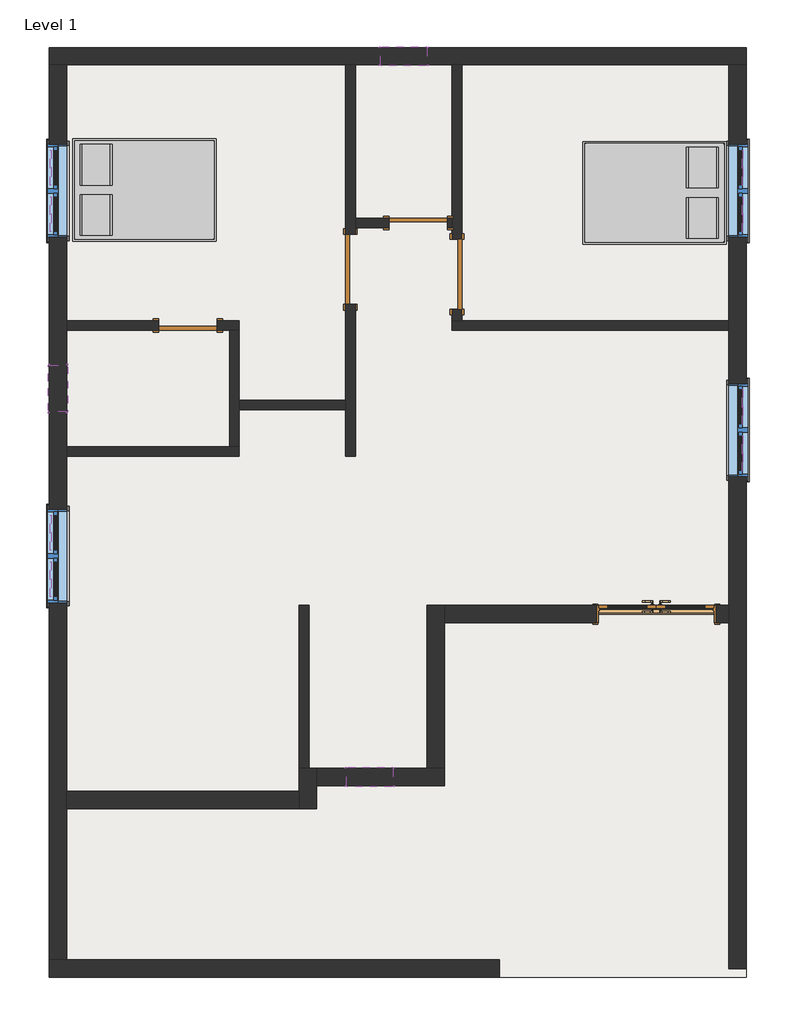
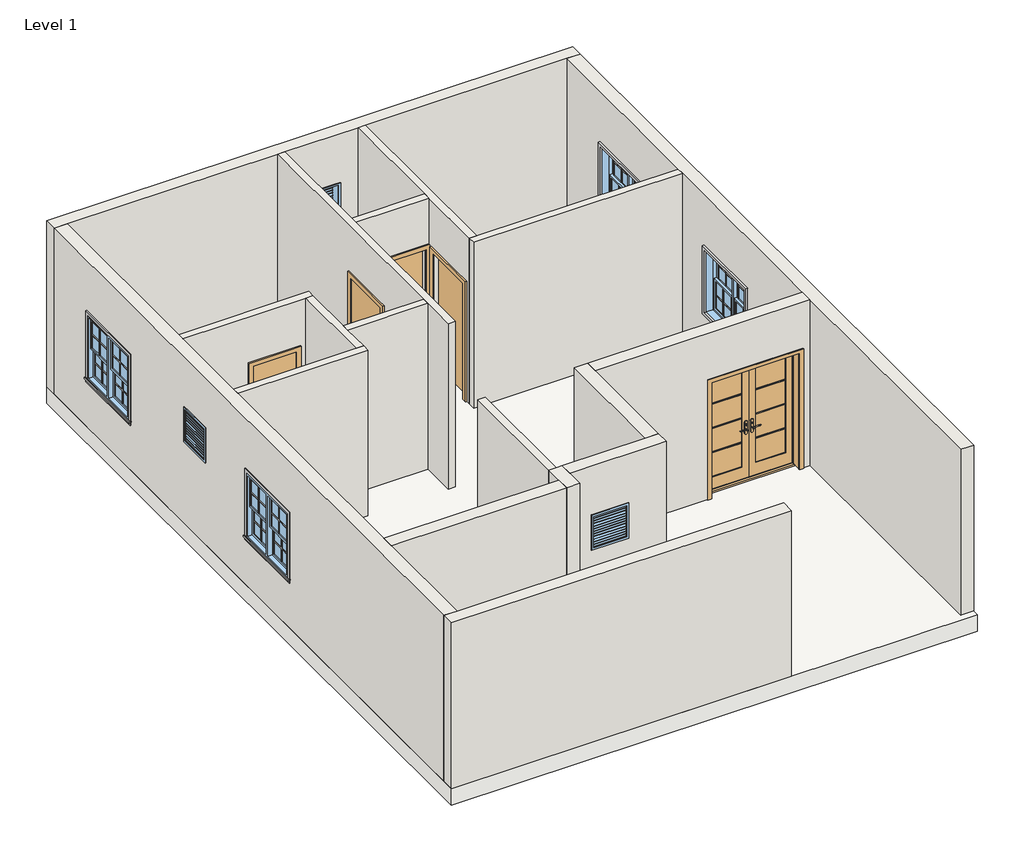
# One storey: 24 proxies, 18 walls, 7 windows, 5 doors, 2 furniture elements, 1 slab.
"""IFC4 building model written with IfcOpenShell, lengths in millimetres."""

from ifc_helpers import new_model, si_unit, frame, origin, origin_with_axes, place, context, project, spatial, polyline, outline, extrude, faceted_brep, transform, mapped, element, save
from components import muntin_pattern_2x2_muntin_pattern_2x2_3e1923be, muntin_pattern_2x2_muntin_pattern_2x2_6213a163, trim_window_exterior_flat_with_sill_91d32942, trim_window_exterior_flat_with_sill_c7d07f6c, trim_window_interior_flat_picture_frame_37b958cc, trim_window_interior_flat_picture_frame_8d0988b3, door_7ffae4ec, door_5304b0a0, door_0715e8d2, door_e36758a9, door_4d6c7550, bed_1_1346_x_1880mm_double_99e58f25, window_e23adcbe, window_25281ba2, window_f2d8fef0, window_407d3824

model = new_model("IFC4")

# Units and contexts
model_context = context("Model", 3, world=origin())
ifc_project = project(units=[si_unit("LENGTHUNIT", "METRE", prefix="MILLI")], contexts=[model_context])

# Site, building, storey
site = spatial("IfcSite", under=ifc_project)
building = spatial("IfcBuilding", under=site)
storey = spatial("IfcBuildingStorey", under=building, Name="Level 1", Elevation=0.0)

# Proxies
placement = place(None, origin())
muntin_pattern_2x2_muntin_pattern_2x2_shape = muntin_pattern_2x2_muntin_pattern_2x2_3e1923be(model_context)
element("IfcBuildingElementProxy", 1, Name="Muntin Pattern_2x2 : Muntin Pattern_2x2", ObjectType="Muntin Pattern_2x2 : Muntin Pattern_2x2", at=placement, inside=storey, context=model_context, shape_type="MappedRepresentation", body=[
    mapped(muntin_pattern_2x2_muntin_pattern_2x2_shape, transform((-10657.2556914, 7698.8778437, 1520.825), x_axis=(0.0, 1.0, 0.0), y_axis=(-1.0, 0.0, 0.0), z_axis=(0.0, 0.0, 1.0))),
])
element("IfcBuildingElementProxy", 2, Name="Muntin Pattern_2x2 : Muntin Pattern_2x2", ObjectType="Muntin Pattern_2x2 : Muntin Pattern_2x2", at=placement, inside=storey, context=model_context, shape_type="MappedRepresentation", body=[
    mapped(muntin_pattern_2x2_muntin_pattern_2x2_shape, transform((-10612.8056914, 7698.8778437, 990.6), x_axis=(0.0, 1.0, 0.0), y_axis=(-1.0, 0.0, 0.0), z_axis=(0.0, 0.0, 1.0))),
])
element("IfcBuildingElementProxy", 3, Name="Muntin Pattern_2x2 : Muntin Pattern_2x2", ObjectType="Muntin Pattern_2x2 : Muntin Pattern_2x2", at=placement, inside=storey, context=model_context, shape_type="MappedRepresentation", body=[
    mapped(muntin_pattern_2x2_muntin_pattern_2x2_shape, transform((-10657.2556914, 2910.9778437, 1520.825), x_axis=(0.0, 1.0, 0.0), y_axis=(-1.0, 0.0, 0.0), z_axis=(0.0, 0.0, 1.0))),
])
element("IfcBuildingElementProxy", 4, Name="Muntin Pattern_2x2 : Muntin Pattern_2x2", ObjectType="Muntin Pattern_2x2 : Muntin Pattern_2x2", at=placement, inside=storey, context=model_context, shape_type="MappedRepresentation", body=[
    mapped(muntin_pattern_2x2_muntin_pattern_2x2_shape, transform((-10612.8056914, 2910.9778437, 990.6), x_axis=(0.0, 1.0, 0.0), y_axis=(-1.0, 0.0, 0.0), z_axis=(0.0, 0.0, 1.0))),
])
element("IfcBuildingElementProxy", 5, Name="Muntin Pattern_2x2 : Muntin Pattern_2x2", ObjectType="Muntin Pattern_2x2 : Muntin Pattern_2x2", at=placement, inside=storey, context=model_context, shape_type="MappedRepresentation", body=[
    mapped(muntin_pattern_2x2_muntin_pattern_2x2_shape, transform((-1583.1056914, 3953.9653437, 1520.825), x_axis=(0.0, -1.0, 0.0), y_axis=(1.0, 0.0, 0.0), z_axis=(0.0, 0.0, 1.0))),
])
element("IfcBuildingElementProxy", 6, Name="Muntin Pattern_2x2 : Muntin Pattern_2x2", ObjectType="Muntin Pattern_2x2 : Muntin Pattern_2x2", at=placement, inside=storey, context=model_context, shape_type="MappedRepresentation", body=[
    mapped(muntin_pattern_2x2_muntin_pattern_2x2_shape, transform((-1627.5556914, 3953.9653437, 990.6), x_axis=(0.0, -1.0, 0.0), y_axis=(1.0, 0.0, 0.0), z_axis=(0.0, 0.0, 1.0))),
])
element("IfcBuildingElementProxy", 7, Name="Muntin Pattern_2x2 : Muntin Pattern_2x2", ObjectType="Muntin Pattern_2x2 : Muntin Pattern_2x2", at=placement, inside=storey, context=model_context, shape_type="MappedRepresentation", body=[
    mapped(muntin_pattern_2x2_muntin_pattern_2x2_shape, transform((-1583.1056914, 7090.8653437, 1520.825), x_axis=(0.0, -1.0, 0.0), y_axis=(1.0, 0.0, 0.0), z_axis=(0.0, 0.0, 1.0))),
])
element("IfcBuildingElementProxy", 8, Name="Muntin Pattern_2x2 : Muntin Pattern_2x2", ObjectType="Muntin Pattern_2x2 : Muntin Pattern_2x2", at=placement, inside=storey, context=model_context, shape_type="MappedRepresentation", body=[
    mapped(muntin_pattern_2x2_muntin_pattern_2x2_shape, transform((-1627.5556914, 7090.8653437, 990.6), x_axis=(0.0, -1.0, 0.0), y_axis=(1.0, 0.0, 0.0), z_axis=(0.0, 0.0, 1.0))),
])
muntin_pattern_2x2_muntin_pattern_2x2_2_shape = muntin_pattern_2x2_muntin_pattern_2x2_6213a163(model_context)
element("IfcBuildingElementProxy", 9, Name="Muntin Pattern_2x2 : Muntin Pattern_2x2", ObjectType="Muntin Pattern_2x2 : Muntin Pattern_2x2", at=placement, inside=storey, context=model_context, shape_type="MappedRepresentation", body=[
    mapped(muntin_pattern_2x2_muntin_pattern_2x2_2_shape, transform((-10657.2556914, 7090.8653437, 1520.825), x_axis=(0.0, -1.0, 0.0), y_axis=(1.0, 0.0, 0.0), z_axis=(0.0, 0.0, 1.0))),
])
element("IfcBuildingElementProxy", 10, Name="Muntin Pattern_2x2 : Muntin Pattern_2x2", ObjectType="Muntin Pattern_2x2 : Muntin Pattern_2x2", at=placement, inside=storey, context=model_context, shape_type="MappedRepresentation", body=[
    mapped(muntin_pattern_2x2_muntin_pattern_2x2_2_shape, transform((-10612.8056914, 7090.8653437, 990.6), x_axis=(0.0, -1.0, 0.0), y_axis=(1.0, 0.0, 0.0), z_axis=(0.0, 0.0, 1.0))),
])
element("IfcBuildingElementProxy", 11, Name="Muntin Pattern_2x2 : Muntin Pattern_2x2", ObjectType="Muntin Pattern_2x2 : Muntin Pattern_2x2", at=placement, inside=storey, context=model_context, shape_type="MappedRepresentation", body=[
    mapped(muntin_pattern_2x2_muntin_pattern_2x2_2_shape, transform((-10657.2556914, 2302.9653437, 1520.825), x_axis=(0.0, -1.0, 0.0), y_axis=(1.0, 0.0, 0.0), z_axis=(0.0, 0.0, 1.0))),
])
element("IfcBuildingElementProxy", 12, Name="Muntin Pattern_2x2 : Muntin Pattern_2x2", ObjectType="Muntin Pattern_2x2 : Muntin Pattern_2x2", at=placement, inside=storey, context=model_context, shape_type="MappedRepresentation", body=[
    mapped(muntin_pattern_2x2_muntin_pattern_2x2_2_shape, transform((-10612.8056914, 2302.9653437, 990.6), x_axis=(0.0, -1.0, 0.0), y_axis=(1.0, 0.0, 0.0), z_axis=(0.0, 0.0, 1.0))),
])
element("IfcBuildingElementProxy", 13, Name="Muntin Pattern_2x2 : Muntin Pattern_2x2", ObjectType="Muntin Pattern_2x2 : Muntin Pattern_2x2", at=placement, inside=storey, context=model_context, shape_type="MappedRepresentation", body=[
    mapped(muntin_pattern_2x2_muntin_pattern_2x2_2_shape, transform((-1583.1056914, 4561.9778437, 1520.825), x_axis=(0.0, 1.0, 0.0), y_axis=(-1.0, 0.0, 0.0), z_axis=(0.0, 0.0, 1.0))),
])
element("IfcBuildingElementProxy", 14, Name="Muntin Pattern_2x2 : Muntin Pattern_2x2", ObjectType="Muntin Pattern_2x2 : Muntin Pattern_2x2", at=placement, inside=storey, context=model_context, shape_type="MappedRepresentation", body=[
    mapped(muntin_pattern_2x2_muntin_pattern_2x2_2_shape, transform((-1627.5556914, 4561.9778437, 990.6), x_axis=(0.0, 1.0, 0.0), y_axis=(-1.0, 0.0, 0.0), z_axis=(0.0, 0.0, 1.0))),
])
element("IfcBuildingElementProxy", 15, Name="Muntin Pattern_2x2 : Muntin Pattern_2x2", ObjectType="Muntin Pattern_2x2 : Muntin Pattern_2x2", at=placement, inside=storey, context=model_context, shape_type="MappedRepresentation", body=[
    mapped(muntin_pattern_2x2_muntin_pattern_2x2_2_shape, transform((-1583.1056914, 7698.8778437, 1520.825), x_axis=(0.0, 1.0, 0.0), y_axis=(-1.0, 0.0, 0.0), z_axis=(0.0, 0.0, 1.0))),
])
element("IfcBuildingElementProxy", 16, Name="Muntin Pattern_2x2 : Muntin Pattern_2x2", ObjectType="Muntin Pattern_2x2 : Muntin Pattern_2x2", at=placement, inside=storey, context=model_context, shape_type="MappedRepresentation", body=[
    mapped(muntin_pattern_2x2_muntin_pattern_2x2_2_shape, transform((-1627.5556914, 7698.8778437, 990.6), x_axis=(0.0, 1.0, 0.0), y_axis=(-1.0, 0.0, 0.0), z_axis=(0.0, 0.0, 1.0))),
])
trim_window_exterior_flat_with_sill_shape = trim_window_exterior_flat_with_sill_91d32942(model_context)
element("IfcBuildingElementProxy", 17, Name="Trim-Window-Exterior-Flat : with Sill", ObjectType="Trim-Window-Exterior-Flat : with Sill", at=placement, inside=storey, context=model_context, shape_type="MappedRepresentation", body=[
    mapped(trim_window_exterior_flat_with_sill_shape, transform((-1548.1806914, 7394.8715937, 2082.8), x_axis=(0.0, 1.0, 0.0), y_axis=(0.0, 0.0, 1.0), z_axis=(1.0, 0.0, 0.0))),
])
trim_window_exterior_flat_with_sill_2_shape = trim_window_exterior_flat_with_sill_c7d07f6c(model_context)
element("IfcBuildingElementProxy", 18, Name="Trim-Window-Exterior-Flat : with Sill", ObjectType="Trim-Window-Exterior-Flat : with Sill", at=placement, inside=storey, context=model_context, shape_type="MappedRepresentation", body=[
    mapped(trim_window_exterior_flat_with_sill_2_shape, transform((-10692.1806914, 7394.8715937, 2082.8), x_axis=(0.0, 1.0, 0.0), y_axis=(0.0, 0.0, -1.0), z_axis=(-1.0, 0.0, 0.0))),
])
element("IfcBuildingElementProxy", 19, Name="Trim-Window-Exterior-Flat : with Sill", ObjectType="Trim-Window-Exterior-Flat : with Sill", at=placement, inside=storey, context=model_context, shape_type="MappedRepresentation", body=[
    mapped(trim_window_exterior_flat_with_sill_2_shape, transform((-10692.1806914, 2606.9715937, 2082.8), x_axis=(0.0, 1.0, 0.0), y_axis=(0.0, 0.0, -1.0), z_axis=(-1.0, 0.0, 0.0))),
])
element("IfcBuildingElementProxy", 20, Name="Trim-Window-Exterior-Flat : with Sill", ObjectType="Trim-Window-Exterior-Flat : with Sill", at=placement, inside=storey, context=model_context, shape_type="MappedRepresentation", body=[
    mapped(trim_window_exterior_flat_with_sill_2_shape, transform((-1548.1806914, 4257.9715937, 2082.8), x_axis=(0.0, -1.0, 0.0), y_axis=(0.0, 0.0, -1.0), z_axis=(1.0, 0.0, 0.0))),
])
trim_window_interior_flat_picture_frame_shape = trim_window_interior_flat_picture_frame_37b958cc(model_context)
element("IfcBuildingElementProxy", 21, Name="Trim-Window-Interior-Flat : Picture Frame", ObjectType="Trim-Window-Interior-Flat : Picture Frame", at=placement, inside=storey, context=model_context, shape_type="MappedRepresentation", body=[
    mapped(trim_window_interior_flat_picture_frame_shape, transform((-1776.7806914, 7394.8715937, 2082.8), x_axis=(0.0, -1.0, 0.0), y_axis=(0.0, 0.0, 1.0), z_axis=(-1.0, 0.0, 0.0))),
])
trim_window_interior_flat_picture_frame_2_shape = trim_window_interior_flat_picture_frame_8d0988b3(model_context)
element("IfcBuildingElementProxy", 22, Name="Trim-Window-Interior-Flat : Picture Frame", ObjectType="Trim-Window-Interior-Flat : Picture Frame", at=placement, inside=storey, context=model_context, shape_type="MappedRepresentation", body=[
    mapped(trim_window_interior_flat_picture_frame_2_shape, transform((-10463.5806914, 7394.8715937, 2082.8), x_axis=(0.0, -1.0, 0.0), y_axis=(0.0, 0.0, -1.0), z_axis=(1.0, 0.0, 0.0))),
])
element("IfcBuildingElementProxy", 23, Name="Trim-Window-Interior-Flat : Picture Frame", ObjectType="Trim-Window-Interior-Flat : Picture Frame", at=placement, inside=storey, context=model_context, shape_type="MappedRepresentation", body=[
    mapped(trim_window_interior_flat_picture_frame_2_shape, transform((-10463.5806914, 2606.9715937, 2082.8), x_axis=(0.0, -1.0, 0.0), y_axis=(0.0, 0.0, -1.0), z_axis=(1.0, 0.0, 0.0))),
])
element("IfcBuildingElementProxy", 24, Name="Trim-Window-Interior-Flat : Picture Frame", ObjectType="Trim-Window-Interior-Flat : Picture Frame", at=placement, inside=storey, context=model_context, shape_type="MappedRepresentation", body=[
    mapped(trim_window_interior_flat_picture_frame_2_shape, transform((-1776.7806914, 4257.9715937, 2082.8), x_axis=(0.0, 1.0, 0.0), y_axis=(0.0, 0.0, -1.0), z_axis=(-1.0, 0.0, 0.0))),
])

# Doors
door_shape = door_7ffae4ec(model_context)
element("IfcDoor", 25, ObjectType="Door-Exterior-Double-Full Glass-Wood_Clad : 60\" x 84\"", at=placement, inside=storey, context=model_context, shape_type="MappedRepresentation", body=[
    mapped(door_shape, transform((-2729.2806914, 1848.1465937, 0.0), x_axis=(1.0, 0.0, 0.0), y_axis=(0.0, 1.0, 0.0), z_axis=(0.0, 0.0, 1.0))),
])
door_2_shape = door_5304b0a0(model_context)
element("IfcDoor", 26, ObjectType="Door-Single-Panel : 36\" x 84\"", at=placement, inside=storey, context=model_context, shape_type="MappedRepresentation", body=[
    mapped(door_2_shape, transform((-6742.4806914, 6366.1715937, 0.0), x_axis=(0.0, -1.0, 0.0), y_axis=(1.0, 0.0, 0.0), z_axis=(0.0, 0.0, 1.0))),
])
door_3_shape = door_0715e8d2(model_context)
element("IfcDoor", 27, ObjectType="Door-Single-Panel : 36\" x 84\"", at=placement, inside=storey, context=model_context, shape_type="MappedRepresentation", body=[
    mapped(door_3_shape, transform((-5345.4806914, 6302.6715937, 0.0), x_axis=(0.0, -1.0, 0.0), y_axis=(1.0, 0.0, 0.0), z_axis=(0.0, 0.0, 1.0))),
])
door_4_shape = door_e36758a9(model_context)
element("IfcDoor", 28, ObjectType="Single-Flush : 30\" x 84\"", at=placement, inside=storey, context=model_context, shape_type="MappedRepresentation", body=[
    mapped(door_4_shape, transform((-8876.0806914, 5629.5715937, 0.0), x_axis=(1.0, 0.0, 0.0), y_axis=(0.0, 1.0, 0.0), z_axis=(0.0, 0.0, 1.0))),
])
door_5_shape = door_4d6c7550(model_context)
element("IfcDoor", 29, ObjectType="Single-Flush : 30\" x 84\"", at=placement, inside=storey, context=model_context, shape_type="MappedRepresentation", body=[
    mapped(door_5_shape, transform((-5853.4806914, 6975.7715937, 0.0), x_axis=(1.0, 0.0, 0.0), y_axis=(0.0, 1.0, 0.0), z_axis=(0.0, 0.0, 1.0))),
])

# Furniture
bed_1_1346_x_1880mm_double_shape = bed_1_1346_x_1880mm_double_99e58f25(model_context)
element("IfcFurniture", 30, ObjectType="Bed (1) : 1346 x 1880mm - Double", at=placement, inside=storey, context=model_context, shape_type="MappedRepresentation", body=[
    mapped(bed_1_1346_x_1880mm_double_shape, transform((-2520.4511832, 7708.5240527, 0.0), x_axis=(0.0, -1.0, 0.0), y_axis=(1.0, 0.0, 0.0), z_axis=(0.0, 0.0, 1.0))),
])
element("IfcFurniture", 31, ObjectType="Bed (1) : 1346 x 1880mm - Double", at=placement, inside=storey, context=model_context, shape_type="MappedRepresentation", body=[
    mapped(bed_1_1346_x_1880mm_double_shape, transform((-9681.8101996, 7068.5191346, 0.0), x_axis=(0.0, 1.0, 0.0), y_axis=(-1.0, 0.0, 0.0), z_axis=(0.0, 0.0, 1.0))),
])

# Slab
element("IfcSlab", 32, ObjectType="Generic - 12\"", at=placement, inside=storey, context=model_context, shape_type="SweptSolid", body=[
    extrude(outline(polyline([(-10692.1806914, 9274.4715937), (-1548.1806914, 9274.4715937), (-1548.1806914, -2917.5284063), (-10692.1806914, -2917.5284063), (-10692.1806914, 9274.4715937)])), frame((0.0, 0.0, -304.8), z_axis=(0.0, 0.0, 1.0), x_axis=(1.0, 0.0, 0.0)), (0.0, 0.0, 1.0), 304.8),
])

# Walls
element("IfcWall", 33, ObjectType="Generic - 5\"", at=placement, inside=storey, context=model_context, shape_type="Brep", body=[
    faceted_brep([(-8495.0806914, 5566.0715937, 2133.6), (-8495.0806914, 5566.0715937, 0.0), (-8329.9806914, 5566.0715937, 0.0), (-8202.9806914, 5566.0715937, 0.0), (-8202.9806914, 5566.0715937, 3048.0), (-8329.9806914, 5566.0715937, 3048.0), (-10463.5806914, 5566.0715937, 3048.0), (-10463.5806914, 5566.0715937, 0.0), (-9257.0806914, 5566.0715937, 0.0), (-9257.0806914, 5566.0715937, 2133.6), (-8202.9806914, 5693.0715937, 0.0), (-8495.0806914, 5693.0715937, 0.0), (-8495.0806914, 5693.0715937, 2133.6), (-9257.0806914, 5693.0715937, 2133.6), (-9257.0806914, 5693.0715937, 0.0), (-10463.5806914, 5693.0715937, 0.0), (-10463.5806914, 5693.0715937, 3048.0), (-8202.9806914, 5693.0715937, 3048.0)], [[[0, 1, 2, 3, 4, 5, 6, 7, 8, 9]], [[10, 11, 12, 13, 14, 15, 16, 17]], [[8, 7, 15, 14]], [[3, 2, 1, 11, 10]], [[6, 5, 4, 17, 16]], [[7, 6, 16, 15]], [[4, 3, 10, 17]], [[12, 11, 1, 0]], [[13, 12, 0, 9]], [[14, 13, 9, 8]]]),
])
element("IfcWall", 34, ObjectType="Generic - 5\"", at=placement, inside=storey, context=model_context, shape_type="Brep", body=[
    faceted_brep([(-6805.9806914, 5908.9715937, 2133.6), (-6805.9806914, 5908.9715937, 0.0), (-6805.9806914, 4651.6715937, 0.0), (-6805.9806914, 4524.6715937, 0.0), (-6805.9806914, 3915.0715937, 0.0), (-6805.9806914, 3915.0715937, 3048.0), (-6805.9806914, 4524.6715937, 3048.0), (-6805.9806914, 4651.6715937, 3048.0), (-6805.9806914, 9045.8715937, 3048.0), (-6805.9806914, 9045.8715937, 0.0), (-6805.9806914, 6823.3715937, 0.0), (-6805.9806914, 6823.3715937, 2133.6), (-6678.9806914, 3915.0715937, 0.0), (-6678.9806914, 5908.9715937, 0.0), (-6678.9806914, 5908.9715937, 2133.6), (-6678.9806914, 6823.3715937, 2133.6), (-6678.9806914, 6823.3715937, 0.0), (-6678.9806914, 6912.2715937, 0.0), (-6678.9806914, 7039.2715937, 0.0), (-6678.9806914, 9045.8715937, 0.0), (-6678.9806914, 9045.8715937, 3048.0), (-6678.9806914, 7039.2715937, 3048.0), (-6678.9806914, 6912.2715937, 3048.0), (-6678.9806914, 3915.0715937, 3048.0)], [[[0, 1, 2, 3, 4, 5, 6, 7, 8, 9, 10, 11]], [[12, 13, 14, 15, 16, 17, 18, 19, 20, 21, 22, 23]], [[10, 9, 19, 18, 17, 16]], [[4, 3, 2, 1, 13, 12]], [[5, 4, 12, 23]], [[8, 7, 6, 5, 23, 22, 21, 20]], [[9, 8, 20, 19]], [[14, 13, 1, 0]], [[15, 14, 0, 11]], [[16, 15, 11, 10]]]),
])
element("IfcWall", 35, ObjectType="Generic - 5\"", at=placement, inside=storey, context=model_context, shape_type="SweptSolid", body=[
    extrude(outline(polyline([(2133.6, -5472.4806914), (0.0, -5472.4806914), (0.0, -5408.9806914), (3048.0, -5408.9806914), (3048.0, -6678.9806914), (0.0, -6678.9806914), (0.0, -6234.4806914), (2133.6, -6234.4806914), (2133.6, -5472.4806914)])), frame((0.0, 6912.2715937, 0.0), z_axis=(0.0, 1.0, 0.0), x_axis=(0.0, 0.0, 1.0)), (0.0, 0.0, 1.0), 127.0),
])
element("IfcWall", 36, ObjectType="Generic - 5\"", at=placement, inside=storey, context=model_context, shape_type="Brep", body=[
    faceted_brep([(-5281.9806914, 5693.0715937, 0.0), (-5281.9806914, 5845.4715937, 0.0), (-5281.9806914, 5845.4715937, 2133.6), (-5281.9806914, 6759.8715937, 2133.6), (-5281.9806914, 6759.8715937, 0.0), (-5281.9806914, 9045.8715937, 0.0), (-5281.9806914, 9045.8715937, 3048.0), (-5281.9806914, 5693.0715937, 3048.0), (-5408.9806914, 5845.4715937, 2133.6), (-5408.9806914, 5845.4715937, 0.0), (-5408.9806914, 5693.0715937, 0.0), (-5408.9806914, 5693.0715937, 3048.0), (-5408.9806914, 6912.2715937, 3048.0), (-5408.9806914, 7039.2715937, 3048.0), (-5408.9806914, 9045.8715937, 3048.0), (-5408.9806914, 9045.8715937, 0.0), (-5408.9806914, 7039.2715937, 0.0), (-5408.9806914, 6912.2715937, 0.0), (-5408.9806914, 6759.8715937, 0.0), (-5408.9806914, 6759.8715937, 2133.6)], [[[0, 1, 2, 3, 4, 5, 6, 7]], [[8, 9, 10, 11, 12, 13, 14, 15, 16, 17, 18, 19]], [[10, 9, 1, 0]], [[18, 17, 16, 15, 5, 4]], [[7, 6, 14, 13, 12, 11]], [[6, 5, 15, 14]], [[0, 7, 11, 10]], [[2, 1, 9, 8]], [[3, 2, 8, 19]], [[4, 3, 19, 18]]]),
])
element("IfcWall", 37, ObjectType="Generic - 5\"", at=placement, inside=storey, context=model_context, shape_type="Brep", body=[
    faceted_brep([(-1776.7806914, 5693.0715937, 0.0), (-5281.9806914, 5693.0715937, 0.0), (-5408.9806914, 5693.0715937, 0.0), (-5408.9806914, 5693.0715937, 3048.0), (-5281.9806914, 5693.0715937, 3048.0), (-1776.7806914, 5693.0715937, 3048.0), (-1776.7806914, 5566.0715937, 0.0), (-1776.7806914, 5566.0715937, 3048.0), (-5408.9806914, 5566.0715937, 3048.0), (-5408.9806914, 5566.0715937, 0.0)], [[[0, 1, 2, 3, 4, 5]], [[6, 7, 8, 9]], [[2, 1, 0, 6, 9]], [[5, 4, 3, 8, 7]], [[0, 5, 7, 6]], [[3, 2, 9, 8]]]),
])
element("IfcWall", 38, ObjectType="Generic - 5\"", at=placement, inside=storey, context=model_context, shape_type="Brep", body=[
    faceted_brep([(-10463.5806914, 3915.0715937, 0.0), (-8202.9806914, 3915.0715937, 0.0), (-8202.9806914, 3915.0715937, 3048.0), (-10463.5806914, 3915.0715937, 3048.0), (-10463.5806914, 4042.0715937, 0.0), (-10463.5806914, 4042.0715937, 3048.0), (-8329.9806914, 4042.0715937, 3048.0), (-8202.9806914, 4042.0715937, 3048.0), (-8202.9806914, 4042.0715937, 0.0), (-8329.9806914, 4042.0715937, 0.0)], [[[0, 1, 2, 3]], [[4, 5, 6, 7, 8, 9]], [[1, 0, 4, 9, 8]], [[3, 2, 7, 6, 5]], [[0, 3, 5, 4]], [[2, 1, 8, 7]]]),
])
element("IfcWall", 39, ObjectType="Generic - 5\"", at=placement, inside=storey, context=model_context, shape_type="Brep", body=[
    faceted_brep([(-8329.9806914, 5566.0715937, 0.0), (-8329.9806914, 4042.0715937, 0.0), (-8329.9806914, 4042.0715937, 3048.0), (-8329.9806914, 5566.0715937, 3048.0), (-8202.9806914, 5566.0715937, 0.0), (-8202.9806914, 5566.0715937, 3048.0), (-8202.9806914, 4651.6715937, 3048.0), (-8202.9806914, 4524.6715937, 3048.0), (-8202.9806914, 4042.0715937, 3048.0), (-8202.9806914, 4042.0715937, 0.0), (-8202.9806914, 4524.6715937, 0.0), (-8202.9806914, 4651.6715937, 0.0)], [[[0, 1, 2, 3]], [[4, 5, 6, 7, 8, 9, 10, 11]], [[1, 0, 4, 11, 10, 9]], [[3, 2, 8, 7, 6, 5]], [[0, 3, 5, 4]], [[2, 1, 9, 8]]]),
])
element("IfcWall", 40, ObjectType="Generic - 5\"", at=placement, inside=storey, context=model_context, shape_type="SweptSolid", body=[
    extrude(outline(polyline([(-6805.9806914, 4524.6715937), (-8202.9806914, 4524.6715937), (-8202.9806914, 4651.6715937), (-6805.9806914, 4651.6715937), (-6805.9806914, 4524.6715937)])), origin_with_axes(), (0.0, 0.0, 1.0), 3048.0),
])
element("IfcWall", 41, ObjectType="Generic - 5\"", at=placement, inside=storey, context=model_context, shape_type="SweptSolid", body=[
    extrude(outline(polyline([(-7415.5806914, -174.3284063), (-7415.5806914, 1959.2715937), (-7288.5806914, 1959.2715937), (-7288.5806914, -174.3284063), (-7415.5806914, -174.3284063)])), origin_with_axes(), (0.0, 0.0, 1.0), 3048.0),
])
element("IfcWall", 42, ObjectType="Generic - 9\"", at=placement, inside=storey, context=model_context, shape_type="Brep", body=[
    faceted_brep([(-10692.1806914, 9045.8715937, 0.0), (-10463.5806914, 9045.8715937, 0.0), (-6805.9806914, 9045.8715937, 0.0), (-6678.9806914, 9045.8715937, 0.0), (-5408.9806914, 9045.8715937, 0.0), (-5281.9806914, 9045.8715937, 0.0), (-1776.7806914, 9045.8715937, 0.0), (-1548.1806914, 9045.8715937, 0.0), (-1548.1806914, 9045.8715937, 3048.0), (-1776.7806914, 9045.8715937, 3048.0), (-5281.9806914, 9045.8715937, 3048.0), (-5408.9806914, 9045.8715937, 3048.0), (-6678.9806914, 9045.8715937, 3048.0), (-6805.9806914, 9045.8715937, 3048.0), (-10463.5806914, 9045.8715937, 3048.0), (-10692.1806914, 9045.8715937, 3048.0), (-5739.1806914, 9045.8715937, 2133.6), (-5739.1806914, 9045.8715937, 1524.0), (-6348.7806914, 9045.8715937, 1524.0), (-6348.7806914, 9045.8715937, 2133.6), (-10692.1806914, 9274.4715937, 0.0), (-10692.1806914, 9274.4715937, 3048.0), (-1548.1806914, 9274.4715937, 3048.0), (-1548.1806914, 9274.4715937, 0.0), (-5739.1806914, 9274.4715937, 2133.6), (-6348.7806914, 9274.4715937, 2133.6), (-6348.7806914, 9274.4715937, 1524.0), (-5739.1806914, 9274.4715937, 1524.0)], [[[0, 1, 2, 3, 4, 5, 6, 7, 8, 9, 10, 11, 12, 13, 14, 15], [16, 17, 18, 19]], [[20, 21, 22, 23], [24, 25, 26, 27]], [[7, 6, 5, 4, 3, 2, 1, 0, 20, 23]], [[15, 14, 13, 12, 11, 10, 9, 8, 22, 21]], [[8, 7, 23, 22]], [[0, 15, 21, 20]], [[17, 16, 24, 27]], [[18, 17, 27, 26]], [[19, 18, 26, 25]], [[16, 19, 25, 24]]]),
])
element("IfcWall", 43, ObjectType="Generic - 9\"", at=placement, inside=storey, context=model_context, shape_type="Brep", body=[
    faceted_brep([(-1776.7806914, 9045.8715937, 0.0), (-1776.7806914, 5693.0715937, 0.0), (-1776.7806914, 5566.0715937, 0.0), (-1776.7806914, 1959.2715937, 0.0), (-1776.7806914, 1730.6715937, 0.0), (-1776.7806914, -2803.2284063, 0.0), (-1776.7806914, -2803.2284063, 3048.0), (-1776.7806914, 1730.6715937, 3048.0), (-1776.7806914, 1959.2715937, 3048.0), (-1776.7806914, 5566.0715937, 3048.0), (-1776.7806914, 5693.0715937, 3048.0), (-1776.7806914, 9045.8715937, 3048.0), (-1776.7806914, 3648.3715937, 2082.8), (-1776.7806914, 3648.3715937, 914.4), (-1776.7806914, 4867.5715937, 914.4), (-1776.7806914, 4867.5715937, 2082.8), (-1776.7806914, 8004.4715937, 2082.8), (-1776.7806914, 6785.2715937, 2082.8), (-1776.7806914, 6785.2715937, 914.4), (-1776.7806914, 8004.4715937, 914.4), (-1548.1806914, 9045.8715937, 0.0), (-1548.1806914, 9045.8715937, 3048.0), (-1548.1806914, -2803.2284063, 3048.0), (-1548.1806914, -2803.2284063, 0.0), (-1548.1806914, 3648.3715937, 2082.8), (-1548.1806914, 4867.5715937, 2082.8), (-1548.1806914, 4867.5715937, 914.4), (-1548.1806914, 3648.3715937, 914.4), (-1548.1806914, 8004.4715937, 2082.8), (-1548.1806914, 8004.4715937, 914.4), (-1548.1806914, 6785.2715937, 914.4), (-1548.1806914, 6785.2715937, 2082.8)], [[[0, 1, 2, 3, 4, 5, 6, 7, 8, 9, 10, 11], [12, 13, 14, 15], [16, 17, 18, 19]], [[20, 21, 22, 23], [24, 25, 26, 27], [28, 29, 30, 31]], [[5, 4, 3, 2, 1, 0, 20, 23]], [[6, 5, 23, 22]], [[11, 10, 9, 8, 7, 6, 22, 21]], [[0, 11, 21, 20]], [[13, 12, 24, 27]], [[14, 13, 27, 26]], [[15, 14, 26, 25]], [[12, 15, 25, 24]], [[29, 28, 16, 19]], [[30, 29, 19, 18]], [[31, 30, 18, 17]], [[28, 31, 17, 16]]]),
])
element("IfcWall", 44, ObjectType="Generic - 9\"", at=placement, inside=storey, context=model_context, shape_type="Brep", body=[
    faceted_brep([(-4786.6806914, -2688.9284063, 0.0), (-10463.5806914, -2688.9284063, 0.0), (-10692.1806914, -2688.9284063, 0.0), (-10692.1806914, -2688.9284063, 3048.0), (-10463.5806914, -2688.9284063, 3048.0), (-4786.6806914, -2688.9284063, 3048.0), (-4786.6806914, -2917.5284063, 0.0), (-4786.6806914, -2917.5284063, 3048.0), (-10692.1806914, -2917.5284063, 3048.0), (-10692.1806914, -2917.5284063, 0.0)], [[[0, 1, 2, 3, 4, 5]], [[6, 7, 8, 9]], [[2, 1, 0, 6, 9]], [[5, 4, 3, 8, 7]], [[0, 5, 7, 6]], [[3, 2, 9, 8]]]),
])
element("IfcWall", 45, ObjectType="Generic - 9\"", at=placement, inside=storey, context=model_context, shape_type="Brep", body=[
    faceted_brep([(-10463.5806914, -2688.9284063, 0.0), (-10463.5806914, -707.7284063, 0.0), (-10463.5806914, -479.1284063, 0.0), (-10463.5806914, 3915.0715937, 0.0), (-10463.5806914, 4042.0715937, 0.0), (-10463.5806914, 5566.0715937, 0.0), (-10463.5806914, 5693.0715937, 0.0), (-10463.5806914, 9045.8715937, 0.0), (-10463.5806914, 9045.8715937, 3048.0), (-10463.5806914, 5693.0715937, 3048.0), (-10463.5806914, 5566.0715937, 3048.0), (-10463.5806914, 4042.0715937, 3048.0), (-10463.5806914, 3915.0715937, 3048.0), (-10463.5806914, -479.1284063, 3048.0), (-10463.5806914, -707.7284063, 3048.0), (-10463.5806914, -2688.9284063, 3048.0), (-10463.5806914, 8004.4715937, 2082.8), (-10463.5806914, 8004.4715937, 914.4), (-10463.5806914, 6785.2715937, 914.4), (-10463.5806914, 6785.2715937, 2082.8), (-10463.5806914, 3216.5715937, 2082.8), (-10463.5806914, 3216.5715937, 914.4), (-10463.5806914, 1997.3715937, 914.4), (-10463.5806914, 1997.3715937, 2082.8), (-10463.5806914, 4499.2715937, 2133.6), (-10463.5806914, 5108.8715937, 2133.6), (-10463.5806914, 5108.8715937, 1524.0), (-10463.5806914, 4499.2715937, 1524.0), (-10692.1806914, -2688.9284063, 0.0), (-10692.1806914, -2688.9284063, 3048.0), (-10692.1806914, 9045.8715937, 3048.0), (-10692.1806914, 9045.8715937, 0.0), (-10692.1806914, 8004.4715937, 2082.8), (-10692.1806914, 6785.2715937, 2082.8), (-10692.1806914, 6785.2715937, 914.4), (-10692.1806914, 8004.4715937, 914.4), (-10692.1806914, 3216.5715937, 2082.8), (-10692.1806914, 1997.3715937, 2082.8), (-10692.1806914, 1997.3715937, 914.4), (-10692.1806914, 3216.5715937, 914.4), (-10692.1806914, 4499.2715937, 2133.6), (-10692.1806914, 4499.2715937, 1524.0), (-10692.1806914, 5108.8715937, 1524.0), (-10692.1806914, 5108.8715937, 2133.6)], [[[0, 1, 2, 3, 4, 5, 6, 7, 8, 9, 10, 11, 12, 13, 14, 15], [16, 17, 18, 19], [20, 21, 22, 23], [24, 25, 26, 27]], [[28, 29, 30, 31], [32, 33, 34, 35], [36, 37, 38, 39], [40, 41, 42, 43]], [[7, 6, 5, 4, 3, 2, 1, 0, 28, 31]], [[15, 14, 13, 12, 11, 10, 9, 8, 30, 29]], [[8, 7, 31, 30]], [[0, 15, 29, 28]], [[17, 16, 32, 35]], [[18, 17, 35, 34]], [[19, 18, 34, 33]], [[16, 19, 33, 32]], [[21, 20, 36, 39]], [[22, 21, 39, 38]], [[23, 22, 38, 37]], [[20, 23, 37, 36]], [[41, 40, 24, 27]], [[42, 41, 27, 26]], [[43, 42, 26, 25]], [[40, 43, 25, 24]]]),
])
element("IfcWall", 46, ObjectType="Generic - 9\"", at=placement, inside=storey, context=model_context, shape_type="SweptSolid", body=[
    extrude(outline(polyline([(-7415.5806914, -707.7284063), (-10463.5806914, -707.7284063), (-10463.5806914, -479.1284063), (-7415.5806914, -479.1284063), (-7415.5806914, -707.7284063)])), origin_with_axes(), (0.0, 0.0, 1.0), 3048.0),
])
element("IfcWall", 47, ObjectType="Generic - 9\"", at=placement, inside=storey, context=model_context, shape_type="Brep", body=[
    faceted_brep([(-7186.9806914, -707.7284063, 0.0), (-7186.9806914, -402.9284063, 0.0), (-7186.9806914, -174.3284063, 0.0), (-7186.9806914, -174.3284063, 3048.0), (-7186.9806914, -402.9284063, 3048.0), (-7186.9806914, -707.7284063, 3048.0), (-7415.5806914, -707.7284063, 0.0), (-7415.5806914, -707.7284063, 3048.0), (-7415.5806914, -479.1284063, 3048.0), (-7415.5806914, -174.3284063, 3048.0), (-7415.5806914, -174.3284063, 0.0), (-7415.5806914, -479.1284063, 0.0), (-7288.5806914, -174.3284063, 0.0), (-7288.5806914, -174.3284063, 3048.0)], [[[0, 1, 2, 3, 4, 5]], [[6, 7, 8, 9, 10, 11]], [[2, 1, 0, 6, 11, 10, 12]], [[5, 4, 3, 13, 9, 8, 7]], [[0, 5, 7, 6]], [[3, 2, 12, 10, 9, 13]]]),
])
element("IfcWall", 48, ObjectType="Generic - 9\"", at=placement, inside=storey, context=model_context, shape_type="Brep", body=[
    faceted_brep([(-7186.9806914, -402.9284063, 0.0), (-5510.5806914, -402.9284063, 0.0), (-5510.5806914, -402.9284063, 3048.0), (-7186.9806914, -402.9284063, 3048.0), (-6793.2806914, -402.9284063, 2133.6), (-6183.6806914, -402.9284063, 2133.6), (-6183.6806914, -402.9284063, 1524.0), (-6793.2806914, -402.9284063, 1524.0), (-7186.9806914, -174.3284063, 0.0), (-7186.9806914, -174.3284063, 3048.0), (-5739.1806914, -174.3284063, 3048.0), (-5510.5806914, -174.3284063, 3048.0), (-5510.5806914, -174.3284063, 0.0), (-5739.1806914, -174.3284063, 0.0), (-6793.2806914, -174.3284063, 2133.6), (-6793.2806914, -174.3284063, 1524.0), (-6183.6806914, -174.3284063, 1524.0), (-6183.6806914, -174.3284063, 2133.6)], [[[0, 1, 2, 3], [4, 5, 6, 7]], [[8, 9, 10, 11, 12, 13], [14, 15, 16, 17]], [[1, 0, 8, 13, 12]], [[3, 2, 11, 10, 9]], [[0, 3, 9, 8]], [[2, 1, 12, 11]], [[15, 14, 4, 7]], [[16, 15, 7, 6]], [[17, 16, 6, 5]], [[14, 17, 5, 4]]]),
])
element("IfcWall", 49, ObjectType="Generic - 9\"", at=placement, inside=storey, context=model_context, shape_type="Brep", body=[
    faceted_brep([(-5510.5806914, -174.3284063, 0.0), (-5510.5806914, 1730.6715937, 0.0), (-5510.5806914, 1959.2715937, 0.0), (-5510.5806914, 1959.2715937, 3048.0), (-5510.5806914, 1730.6715937, 3048.0), (-5510.5806914, -174.3284063, 3048.0), (-5739.1806914, -174.3284063, 0.0), (-5739.1806914, -174.3284063, 3048.0), (-5739.1806914, 1959.2715937, 3048.0), (-5739.1806914, 1959.2715937, 0.0)], [[[0, 1, 2, 3, 4, 5]], [[6, 7, 8, 9]], [[2, 1, 0, 6, 9]], [[5, 4, 3, 8, 7]], [[0, 5, 7, 6]], [[3, 2, 9, 8]]]),
])
element("IfcWall", 50, ObjectType="Generic - 9\"", at=placement, inside=storey, context=model_context, shape_type="SweptSolid", body=[
    extrude(outline(polyline([(3048.0, -1776.7806914), (3048.0, -5510.5806914), (0.0, -5510.5806914), (0.0, -3516.6806914), (2159.0, -3516.6806914), (2159.0, -1941.8806914), (0.0, -1941.8806914), (0.0, -1776.7806914), (3048.0, -1776.7806914)])), frame((0.0, 1730.6715937, 0.0), z_axis=(0.0, 1.0, 0.0), x_axis=(0.0, 0.0, 1.0)), (0.0, 0.0, 1.0), 228.6),
])

# Windows
window_shape = window_e23adcbe(model_context)
element("IfcWindow", 51, ObjectType="Window-Double-Hung-Double : 48\" x 46\"", at=placement, inside=storey, context=model_context, shape_type="MappedRepresentation", body=[
    mapped(window_shape, transform((-1662.4806914, 7394.8715937, 0.0), x_axis=(0.0, -1.0, 0.0), y_axis=(1.0, 0.0, 0.0), z_axis=(0.0, 0.0, 1.0))),
])
window_2_shape = window_25281ba2(model_context)
element("IfcWindow", 52, ObjectType="Window-Double-Hung-Double : 48\" x 46\"", at=placement, inside=storey, context=model_context, shape_type="MappedRepresentation", body=[
    mapped(window_2_shape, transform((-10577.8806914, 7394.8715937, 0.0), x_axis=(0.0, -1.0, 0.0), y_axis=(1.0, 0.0, 0.0), z_axis=(0.0, 0.0, 1.0))),
])
element("IfcWindow", 53, ObjectType="Window-Double-Hung-Double : 48\" x 46\"", at=placement, inside=storey, context=model_context, shape_type="MappedRepresentation", body=[
    mapped(window_2_shape, transform((-10577.8806914, 2606.9715937, 0.0), x_axis=(0.0, -1.0, 0.0), y_axis=(1.0, 0.0, 0.0), z_axis=(0.0, 0.0, 1.0))),
])
element("IfcWindow", 54, ObjectType="Window-Double-Hung-Double : 48\" x 46\"", at=placement, inside=storey, context=model_context, shape_type="MappedRepresentation", body=[
    mapped(window_2_shape, transform((-1662.4806914, 4257.9715937, 0.0), x_axis=(0.0, 1.0, 0.0), y_axis=(-1.0, 0.0, 0.0), z_axis=(0.0, 0.0, 1.0))),
])
window_3_shape = window_f2d8fef0(model_context)
element("IfcWindow", 55, ObjectType="Window-Louvers : 24\" x 24\"", at=placement, inside=storey, context=model_context, shape_type="MappedRepresentation", body=[
    mapped(window_3_shape, transform((-10584.2306914, 4804.0715937, 609.6), x_axis=(0.0, 1.0, 0.0), y_axis=(-1.0, 0.0, 0.0), z_axis=(0.0, 0.0, 1.0))),
])
window_4_shape = window_407d3824(model_context)
element("IfcWindow", 56, ObjectType="Window-Louvers : 24\" x 24\"", at=placement, inside=storey, context=model_context, shape_type="MappedRepresentation", body=[
    mapped(window_4_shape, transform((-6043.9806914, 9166.5215937, 609.6), x_axis=(-1.0, 0.0, 0.0), y_axis=(0.0, -1.0, 0.0), z_axis=(0.0, 0.0, 1.0))),
])
element("IfcWindow", 57, ObjectType="Window-Louvers : 24\" x 24\"", at=placement, inside=storey, context=model_context, shape_type="MappedRepresentation", body=[
    mapped(window_4_shape, transform((-6488.4806914, -294.9784063, 609.6), x_axis=(1.0, 0.0, 0.0), y_axis=(0.0, 1.0, 0.0), z_axis=(0.0, 0.0, 1.0))),
])

save(model, "model.ifc")

# Revit data of these elements
# Type "Muntin Pattern_2x2 : Muntin Pattern_2x2"
#   Width [instance default] = 4' - 0"
#   Thickness = 0' - 0 1/2"
#   Height [instance default] = 4' - 0"
#   Distance = 0' - 0 3/4"
#   Interior Material [instance default] = none
#   Exterior Material [instance default] = none
#   Default Elevation = 0
# Type "Trim-Window-Exterior-Flat : with Sill"
#   Trim Width = 0' - 2 1/4"
#   Trim Thickness_Picture Frame = 0' - 1 1/4"
#   Trim Thickness_with Sill = 0' - 0 3/4"
#   Sill Thickness = 0' - 1 1/4"
#   Opening Width [instance default] = 2' - 0"
#   Opening Height [instance default] = 3' - 0"
#   Default Elevation = 4' - 0"
#   Sill = yes
#   Picture Frame = no
#   Trim Material [instance default] = none
# Type "Trim-Window-Interior-Flat : Picture Frame"
#   Trim Thickness_Picture Frame = 0' - 1 1/4"
#   Trim Width = 0' - 2 1/4"
#   Trim Thickness_with Sill = 0' - 0 3/4"
#   Sill Thickness = 0' - 1 1/4"
#   Opening Width [instance default] = 2' - 0"
#   Opening Height [instance default] = 3' - 0"
#   Default Elevation = 4' - 0"
#   Sill = no
#   Picture Frame = yes
#   Trim Material [instance default] = none
# Type "Door-Exterior-Double-Full Glass-Wood_Clad : 60\" x 84\""
#   Type Mark = "9"
#   Assembly Code = "B2030100"
#   Analytic Construction = "French door, wood frame with double glass"
#   Top Rail = 0' - 4 11/16"
#   Threshold Offset [instance default] = 0' - 0 1/2"
#   Thickness = 0' - 1 3/8"
#   Thermal Resistance (R) = 1.9158 (h·ft²·°F)/BTU
#   Swing Angle [instance default] = 90.00°
#   Stiles = 0' - 4 3/4"
#   Rough Width = 5' - 2"
#   Rough Height = 7' - 1"
#   Panel Width = 2' - 6"
#   Door Offset [instance default] = 0' - 0"
#   Height = 7' - 0"
#   Width = 5' - 0"
#   Heat Transfer Coefficient (U) = 0.5220 BTU/(h·ft²·°F)
#   Bottom Rail = 0' - 9 1/8"
#   Exterior Trim [instance default] = yes
#   Threshold [instance default] = yes
#   Show Grill [instance default] = yes
#   Function = 1
#   Trim Material = Cherry
#   Threshold Material = Cherry
#   Panel Material = Cherry
#   Glazing = Glass
#   Frame Material = Cherry
#   Door Handle Material = Aluminum
#   Visual Light Transmittance = 0
#   Solar Heat Gain Coefficient = 0
#   Wall Closure = (empty or 0)
#   Construction Type = (empty or 0)
# Type "Door-Single-Panel : 36\" x 84\""
#   Type Mark = "8"
#   Construction Type Id = "DOOR"
#   Assembly Code = "C1020300"
#   Analytic Construction = "Wooden"
#   Thickness = 0' - 2"
#   Thermal Resistance (R) = 2.5876 (h·ft²·°F)/BTU
#   Swing Angle [instance default] = 90.00°
#   Heat Transfer Coefficient (U) = 0.3865 BTU/(h·ft²·°F)
#   Height = 7' - 0"
#   Trim Projection Ext = 0' - 1"
#   Trim Projection Int = 0' - 1"
#   Trim Width = 0' - 3"
#   Width = 3' - 0"
#   Define Thermal Properties by = 1
#   Panel Material = Wood - Birch - Solid Stained Light Low Gloss
#   Trim Material = Paint - Sienna
#   Visual Light Transmittance = 0
#   Solar Heat Gain Coefficient = 0
#   Function = (empty or 0)
#   Wall Closure = (empty or 0)
# Type "Single-Flush : 30\" x 84\""
#   Type Mark = "4"
#   Construction Type Id = "MDOOR"
#   Assembly Code = "C1020"
#   Analytic Construction = "Metal"
#   Thickness = 0' - 2"
#   Heat Transfer Coefficient (U) = 0.651978 BTU/(h·ft²·°F)
#   Height = 7' - 0"
#   Trim Projection Ext = 0' - 1"
#   Trim Projection Int = 0' - 1"
#   Trim Width = 0' - 3"
#   Width = 2' - 6"
#   Define Thermal Properties by = 1
#   Define Thermal Properties by = 1
#   Door Material = Door - Panel
#   Frame Material = Door - Frame
#   Visual Light Transmittance = 0
#   Solar Heat Gain Coefficient = 0
#   Function = (empty or 0)
#   Wall Closure = (empty or 0)
# Type "Bed (1) : 1346 x 1880mm - Double"
#   Keynote = "N"
#   Length = 6' - 2.01575"
#   Width = 4' - 4.99213"
#   Material Frame = Wood - Birch
#   Material Mattress = Textile - White
#   Default Elevation = 0
# Type "Generic - 12\""
#   Assembly Code = "B1010"
#   Function = 0
#   Layers, outside or top first: 1' - 0" no material (function 1)
# Type "Generic - 5\""
#   Assembly Code = "B2010"
#   Layers, outside or top first: 0' - 5" no material (function 1)
# Type "Generic - 9\""
#   Assembly Code = "B2010"
#   Layers, outside or top first: 0' - 9" no material (function 1)
# Type "Window-Double-Hung-Double : 48\" x 46\""
#   Type Mark = "21"
#   Fire Rating = "0.5h"
#   Construction Type Id = "DG-DR"
#   Assembly Code = "B2020100"
#   Analytic Construction = "Double glazing - domestic"
#   Wall Thickness [instance default] = 0' - 6"
#   Window Inset [instance default] = 0' - 0"
#   Visual Light Transmittance = 0.81
#   Thermal Resistance (R) = 1.8146 (h·ft²·°F)/BTU
#   Solar Heat Gain Coefficient = 0.76
#   Muntin Width = 1' - 6 1/16"
#   Muntin Height = 1' - 7 1/8"
#   Interior Wall Closure [instance default] = 0' - 1 1/2"
#   Rough Width = 4' - 0 1/2"
#   Rough Height = 3' - 10 1/2"
#   Frame Extension [instance default] = 0' - 1 1/4"
#   Exterior Wall Closure [instance default] = 0' - 0 1/2"
#   Extension Jamb [instance default] = 0' - 1 1/2"
#   Heat Transfer Coefficient (U) = 0.5511 BTU/(h·ft²·°F)
#   Height = 3' - 10"
#   Width = 4' - 0"
#   Top Muntin Visibility = yes
#   Indicator Visibility [instance default] = yes
#   Extension Jamb Visibility [instance default] = yes
#   Interior Trim Visibility [instance default] = yes
#   Exterior Trim Visibility [instance default] = yes
#   Define Thermal Properties by = 1
#   Bottom Muntin Visibility = yes
#   Muntin Pattern = Muntin Pattern_2x2 : Muntin Pattern_2x2
#   Interior Trim Material = Wood - Stained
#   Interior Trim = Trim-Window-Interior-Flat : Picture Frame
#   Exterior Trim Material = Clad - White
#   Exterior Trim = Trim-Window-Exterior-Flat : with Sill
#   Glass Panel Material = Glass
#   Exterior Frame Material = Clad - White
#   Interior Frame Material = Wood - Stained
#   Wall Closure = (empty or 0)
# Type "Window-Louvers : 24\" x 24\""
#   Type Mark = "22"
#   Construction Type Id = "GSP4R"
#   Assembly Code = "B20"
#   Analytic Construction = "1/8 in Pilkington single glazing"
#   Visual Light Transmittance = 0.9
#   Thermal Resistance (R) = 1.53941 (h·ft²·°F)/BTU
#   Solar Heat Gain Coefficient = 0.78
#   Max Height = 1' - 11.74264"
#   Height = 2' - 0"
#   Heat Transfer Coefficient (U) = 0.6496 BTU/(h·ft²·°F)
#   Blade Width [instance default] = 1' - 10 1/2"
#   Blade Vertical Thickness = 0' - 0.35355"
#   Blade Thickness = 0' - 0 1/4"
#   Blade Spacing = 0' - 1 1/2"
#   Blade Height = 0' - 1.85355"
#   Blade Depth = 0' - 3"
#   Blade Angle = 45.00°
#   Default Sill Height = 3' - 0"
#   Trim Projection_Exterior = 0' - 0 1/2"
#   Trim Projection_Interior = 0' - 0 1/2"
#   Trim Width_Exterior = 0' - 1 1/2"
#   Trim Width_Interior = 0' - 1 1/2"
#   Width = 2' - 0"
#   Max Blade Count = 12
#   Define Thermal Properties by = 1
#   Blade Count = 12
#   Frame Material = Birch
#   Louver Material = Birch
#   Trim Exterior Material = Birch
#   Trim Interior Material = Birch
#   Wall Closure = (empty or 0)
# Elements 1, 2, 3, 4, 5, 6, 7, 8, 9, 10, 11, 12, 13, 14, 15, 16 (IfcBuildingElementProxy, "Muntin Pattern_2x2 : Muntin Pattern_2x2")
#   Width = 1' - 6 1/16"
#   Height = 1' - 7 1/8"
#   Interior Material = Wood - Stained
#   Exterior Material = Clad - White
#   Phase Created = New Construction
#   Materials on its faces: "Clad - White", "Wood - Stained"
# Elements 17, 18, 19, 20 (IfcBuildingElementProxy, "Trim-Window-Exterior-Flat : with Sill")
#   Opening Width = 4' - 0"
#   Opening Height = 3' - 10"
#   Trim Material = Clad - White
#   Phase Created = New Construction
#   Materials on its faces: "Clad - White"
# Elements 21, 22, 23, 24 (IfcBuildingElementProxy, "Trim-Window-Interior-Flat : Picture Frame")
#   Opening Width = 4' - 0"
#   Opening Height = 3' - 10"
#   Trim Material = Wood - Stained
#   Phase Created = New Construction
#   Materials on its faces: "Wood - Stained"
# Element 25 (IfcDoor, "Door-Exterior-Double-Full Glass-Wood_Clad : 60\" x 84\"")
#   Threshold Offset = 0' - 0 1/2"
#   Swing Angle = 90.00°
#   Door Offset = 0' - 0"
#   Threshold = yes
#   Show Grill = yes
#   Exterior Trim = yes
#   Phase Created = New Construction
#   Materials on its faces: "Cherry", "Aluminum", "Glass"
# Elements 26, 27 (IfcDoor, "Door-Single-Panel : 36\" x 84\"")
#   Swing Angle = 90.00°
#   Phase Created = New Construction
#   Materials on its faces: "Paint - Sienna", "Wood - Birch - Solid Stained Light Low Gloss"
# Elements 28, 29 (IfcDoor, "Single-Flush : 30\" x 84\"")
#   Phase Created = New Construction
#   Materials on its faces: "Door - Frame", "Door - Panel"
# Elements 30, 31 (IfcFurniture, "Bed (1) : 1346 x 1880mm - Double")
#   Phase Created = New Construction
#   Materials on its faces: "Wood - Birch", "Textile - White"
# Element 32 (IfcSlab, "Generic - 12\"")
#   built-in parameter 1001955 = 3.14159 (stored number, unit not read)
#   Height Offset From Level = 0' - 0"
#   Phase Created = New Construction
#   Materials on its faces: "Default Floor"
# Elements 33, 34, 35, 36, 37, 38, 39, 40, 41 (IfcWall, "Generic - 5\"")
#   Top Offset = 0' - 0"
#   Base Offset = 0' - 0"
#   wall height = 10' - 0"
#   Phase Created = New Construction
#   Base Constraint = Level 1
#   Top Constraint = Level 2
#   Materials on its faces: "Default Wall"
# Elements 42, 43, 44, 45, 46, 47, 48, 49, 50 (IfcWall, "Generic - 9\"")
#   Top Offset = 0' - 0"
#   Base Offset = 0' - 0"
#   wall height = 10' - 0"
#   Phase Created = New Construction
#   Base Constraint = Level 1
#   Top Constraint = Level 2
#   Materials on its faces: "Default Wall"
# Element 51 (IfcWindow, "Window-Double-Hung-Double : 48\" x 46\"")
#   Mark = "4"
#   Window Inset = 0' - 0"
#   Interior Wall Closure = 0' - 1 1/2"
#   Frame Extension = 0' - 1 1/4"
#   Exterior Wall Closure = 0' - 0 1/2"
#   Interior Trim Visibility = yes
#   Indicator Visibility = yes
#   Exterior Trim Visibility = yes
#   Phase Created = New Construction
#   Materials on its faces: "Wood - Stained", "Glass", "Clad - White"
# Element 52 (IfcWindow, "Window-Double-Hung-Double : 48\" x 46\"")
#   Mark = "1"
#   Window Inset = 0' - 0"
#   Interior Wall Closure = 0' - 1 1/2"
#   Frame Extension = 0' - 1 1/4"
#   Exterior Wall Closure = 0' - 0 1/2"
#   Interior Trim Visibility = yes
#   Indicator Visibility = yes
#   Exterior Trim Visibility = yes
#   Phase Created = New Construction
#   Materials on its faces: "Wood - Stained", "Glass", "Clad - White"
# Element 53 (IfcWindow, "Window-Double-Hung-Double : 48\" x 46\"")
#   Mark = "2"
#   Window Inset = 0' - 0"
#   Interior Wall Closure = 0' - 1 1/2"
#   Frame Extension = 0' - 1 1/4"
#   Exterior Wall Closure = 0' - 0 1/2"
#   Interior Trim Visibility = yes
#   Indicator Visibility = yes
#   Exterior Trim Visibility = yes
#   Phase Created = New Construction
#   Materials on its faces: "Wood - Stained", "Glass", "Clad - White"
# Element 54 (IfcWindow, "Window-Double-Hung-Double : 48\" x 46\"")
#   Mark = "3"
#   Window Inset = 0' - 0"
#   Interior Wall Closure = 0' - 1 1/2"
#   Frame Extension = 0' - 1 1/4"
#   Exterior Wall Closure = 0' - 0 1/2"
#   Interior Trim Visibility = yes
#   Indicator Visibility = yes
#   Exterior Trim Visibility = yes
#   Phase Created = New Construction
#   Materials on its faces: "Wood - Stained", "Glass", "Clad - White"
# Element 55 (IfcWindow, "Window-Louvers : 24\" x 24\"")
#   Mark = "7"
#   Blade Width = 1' - 10 1/2"
#   Phase Created = New Construction
#   Materials on its faces: "Birch"
# Element 56 (IfcWindow, "Window-Louvers : 24\" x 24\"")
#   Mark = "5"
#   Blade Width = 1' - 10 1/2"
#   Phase Created = New Construction
#   Materials on its faces: "Birch"
# Element 57 (IfcWindow, "Window-Louvers : 24\" x 24\"")
#   Mark = "6"
#   Blade Width = 1' - 10 1/2"
#   Phase Created = New Construction
#   Materials on its faces: "Birch"
# Materials
#   "Cherry": class "Wood", colour RGB 226 177 128, transparency 0, Description = "Prunus Serotina", Cost = 0
#   "Glass": class "Glass", colour RGB 0 128 192, transparency 0.75, Description = "Soda Lime Glass", Cost = 0
#   "Aluminum": class "Metal", colour RGB 247 247 247, transparency 0, Description = "Aluminum 6061", Cost = 0
#   "Wood - Birch - Solid Stained Light Low Gloss": class "Wood", colour RGB 210 159 95, transparency 0, Cost = 0
#   "Paint - Sienna": colour RGB 118 70 51, transparency 0, Cost = 0
#   "Door - Panel": class "Wood", colour RGB 210 159 95, transparency 0, Cost = 0
#   "Door - Frame": colour RGB 118 70 51, transparency 0, Cost = 0
#   "Wood - Birch": colour RGB 224 178 126, transparency 0
#   "Textile - White": colour RGB 247 247 239, transparency 0
#   "Wood - Stained": class "Wood", colour RGB 224 178 126, transparency 0, Cost = 0
#   "Clad - White": class "Wood", colour RGB 242 242 238, transparency 0, Cost = 0
#   "Birch": class "Wood", colour RGB 224 178 126, transparency 0, Description = "Betula Alleghaniensis", Cost = 0
#   "Default Floor": colour RGB 128 128 128, transparency 0, Cost = 0
#   "Default Wall": colour RGB 128 128 128, transparency 0, Cost = 0
